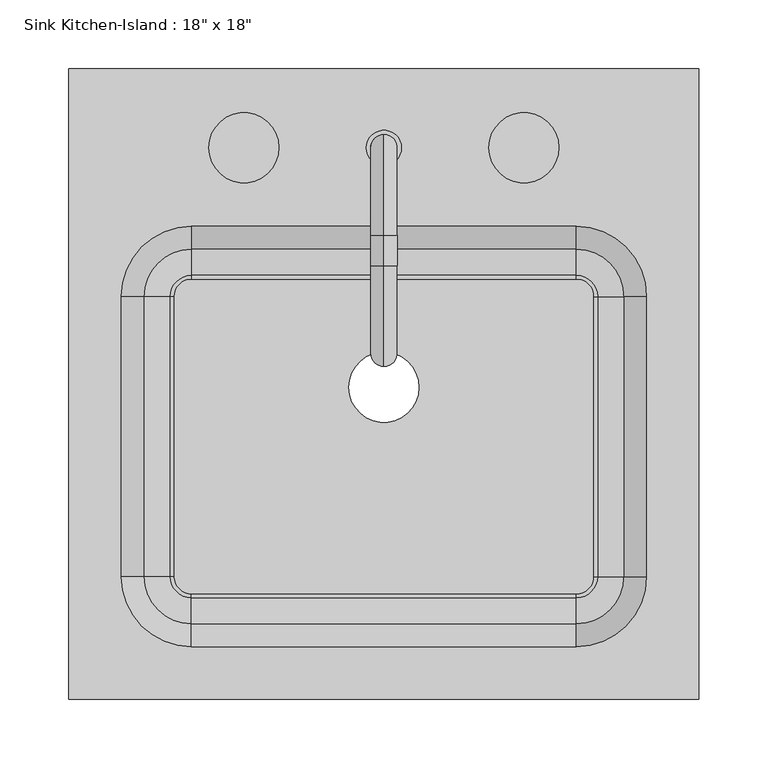
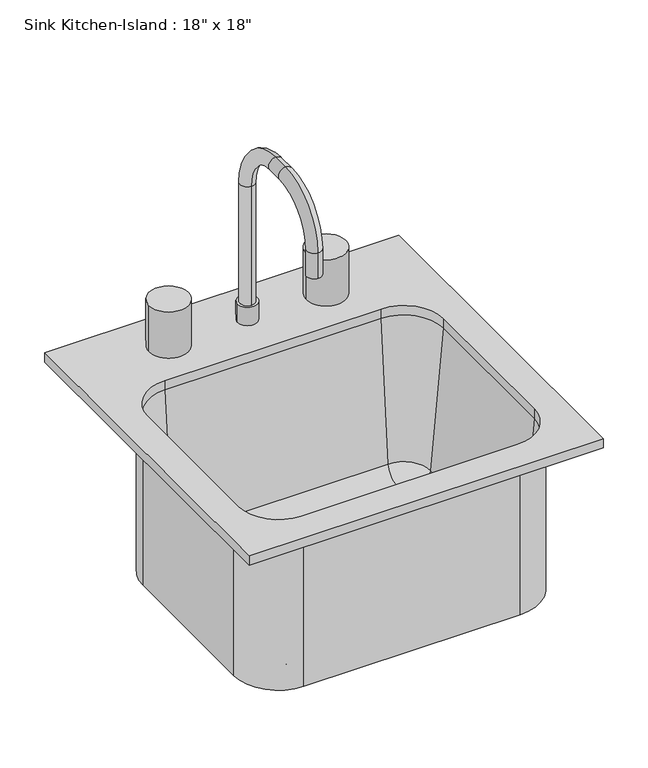
"""IFC4 building model written with IfcOpenShell, lengths in millimetres: flow terminal geometry."""

from ifc_helpers import new_model, si_unit, point, frame, frame_2d, origin, place, context, project, spatial, polyline, circle_curve, ellipse_curve, trimmed, segment, composite_curve, outline, extrude, source, transform, mapped, element, save
from ifc_brep_helpers import plane_surface, cylinder_surface, revolved_surface, advanced_brep


def flow_terminal_871c2e40(model_context):
    return source(origin(), model_context, "Body", "SolidModel", [
        advanced_brep(
        [(244.2892406, 230.9454011, 927.1), (-212.9107594, 230.9454011, 927.1), (-212.9107594, -226.2545989, 927.1), (244.2892406, -226.2545989, 927.1), (155.3892406, 116.6454011, 927.1), (206.1892406, 65.8454011, 927.1), (206.1892406, -137.3545989, 927.1), (155.3892406, -188.1545989, 927.1), (-124.0107594, -188.1545989, 927.1), (-174.8107594, -137.3545989, 927.1), (-174.8107594, 65.8454011, 927.1), (-124.0107594, 116.6454011, 927.1), (244.2892406, 230.9454011, 914.4), (244.2892406, -226.2545989, 914.4), (-212.9107594, -226.2545989, 914.4), (-212.9107594, 230.9454011, 914.4), (212.5392406, 65.8454011, 914.4), (155.3892406, 122.9954011, 914.4), (-124.0107594, 122.9954011, 914.4), (-181.1607594, 65.8454011, 914.4), (-181.1607594, -137.3545989, 914.4), (-124.0107594, -194.5045989, 914.4), (155.3892406, -194.5045989, 914.4), (212.5392406, -137.3545989, 914.4), (155.3892406, 116.6454011, 914.4), (206.1892406, 65.8454011, 914.4), (206.1892406, -137.3545989, 914.4), (155.3892406, -188.1545989, 914.4), (-124.0107594, -188.1545989, 914.4), (-174.8107594, -137.3545989, 914.4), (-174.8107594, 65.8454011, 914.4), (-124.0107594, 116.6454011, 914.4), (212.5392406, 65.8454011, 698.5), (155.3892406, 122.9954011, 698.5), (168.0892406, 65.8454011, 698.5), (155.3892406, 78.5454011, 698.5), (168.0892406, 65.8454011, 708.025), (155.3892406, 78.5454011, 708.025), (170.6776588, 65.8454011, 708.025), (155.3892406, 81.1338193, 708.025), (189.6551678, 65.8454011, 725.4146831), (155.3892406, 100.1113283, 725.4146831), (212.5392406, -137.3545989, 698.5), (168.0892406, -137.3545989, 698.5), (168.0892406, -137.3545989, 708.025), (170.6776588, -137.3545989, 708.025), (189.6551678, -137.3545989, 725.4146831), (155.3892406, -194.5045989, 698.5), (155.3892406, -150.0545989, 698.5), (155.3892406, -150.0545989, 708.025), (155.3892406, -152.6430171, 708.025), (155.3892406, -171.6205261, 725.4146831), (-124.0107594, -194.5045989, 698.5), (-124.0107594, -150.0545989, 698.5), (-124.0107594, -150.0545989, 708.025), (-124.0107594, -152.6430171, 708.025), (-124.0107594, -171.6205261, 725.4146831), (-181.1607594, -137.3545989, 698.5), (-136.7107594, -137.3545989, 698.5), (-136.7107594, -137.3545989, 708.025), (-139.2991776, -137.3545989, 708.025), (-158.2766866, -137.3545989, 725.4146831), (-181.1607594, 65.8454011, 698.5), (-136.7107594, 65.8454011, 698.5), (-136.7107594, 65.8454011, 708.025), (-139.2991776, 65.8454011, 708.025), (-158.2766866, 65.8454011, 725.4146831), (-124.0107594, 122.9954011, 698.5), (-124.0107594, 78.5454011, 698.5), (-124.0107594, 78.5454011, 708.025), (-124.0107594, 81.1338193, 708.025), (-124.0107594, 100.1113283, 725.4146831)],
        [
            (0, 1),
            (1, 2),
            (2, 3),
            (3, 0),
            (4, 5, circle_curve(frame((155.3892406, 65.8454011, 927.1), z_axis=(0.0, 0.0, -1.0), x_axis=(1.0, 0.0, 0.0)), 50.8)),
            (5, 6),
            (6, 7, circle_curve(frame((155.3892406, -137.3545989, 927.1), z_axis=(0.0, 0.0, -1.0), x_axis=(1.0, 0.0, 0.0)), 50.8)),
            (7, 8),
            (8, 9, circle_curve(frame((-124.0107594, -137.3545989, 927.1), z_axis=(0.0, 0.0, -1.0), x_axis=(1.0, 0.0, 0.0)), 50.8)),
            (9, 10),
            (10, 11, circle_curve(frame((-124.0107594, 65.8454011, 927.1), z_axis=(0.0, 0.0, -1.0), x_axis=(1.0, 0.0, 0.0)), 50.8)),
            (11, 4),
            (12, 13),
            (13, 14),
            (14, 15),
            (15, 12),
            (16, 17, circle_curve(frame((155.3892406, 65.8454011, 914.4), z_axis=(0.0, 0.0, 1.0), x_axis=(0.0, 1.0, 0.0)), 57.15)),
            (17, 18),
            (18, 19, circle_curve(frame((-124.0107594, 65.8454011, 914.4), z_axis=(0.0, 0.0, 1.0), x_axis=(-1.0, 0.0, 0.0)), 57.15)),
            (19, 20),
            (20, 21, circle_curve(frame((-124.0107594, -137.3545989, 914.4), z_axis=(0.0, 0.0, 1.0), x_axis=(0.0, -1.0, 0.0)), 57.15)),
            (21, 22),
            (22, 23, circle_curve(frame((155.3892406, -137.3545989, 914.4), z_axis=(0.0, 0.0, 1.0), x_axis=(1.0, 0.0, 0.0)), 57.15)),
            (23, 16),
            (0, 12),
            (15, 1),
            (14, 2),
            (13, 3),
            (4, 24),
            (24, 25, circle_curve(frame((155.3892406, 65.8454011, 914.4), z_axis=(0.0, 0.0, -1.0), x_axis=(1.0, 0.0, 0.0)), 50.8)),
            (25, 5),
            (25, 26),
            (26, 6),
            (26, 27, circle_curve(frame((155.3892406, -137.3545989, 914.4), z_axis=(0.0, 0.0, -1.0), x_axis=(1.0, 0.0, 0.0)), 50.8)),
            (27, 7),
            (27, 28),
            (28, 8),
            (28, 29, circle_curve(frame((-124.0107594, -137.3545989, 914.4), z_axis=(0.0, 0.0, -1.0), x_axis=(1.0, 0.0, 0.0)), 50.8)),
            (29, 9),
            (29, 30),
            (30, 10),
            (30, 31, circle_curve(frame((-124.0107594, 65.8454011, 914.4), z_axis=(0.0, 0.0, -1.0), x_axis=(1.0, 0.0, 0.0)), 50.8)),
            (31, 11),
            (31, 24),
            (32, 33, circle_curve(frame((155.3892406, 65.8454011, 698.5), z_axis=(0.0, 0.0, 1.0), x_axis=(0.0, 1.0, 0.0)), 57.15)),
            (33, 17),
            (16, 32),
            (32, 34),
            (34, 35, circle_curve(frame((155.3892406, 65.8454011, 698.5), z_axis=(0.0, 0.0, 1.0), x_axis=(0.0, 1.0, 0.0)), 12.7)),
            (35, 33),
            (34, 36),
            (36, 37, circle_curve(frame((155.3892406, 65.8454011, 708.025), z_axis=(0.0, 0.0, 1.0), x_axis=(0.0, 1.0, 0.0)), 12.7)),
            (37, 35),
            (36, 38),
            (38, 39, circle_curve(frame((155.3892406, 65.8454011, 708.025), z_axis=(0.0, 0.0, 1.0), x_axis=(0.0, 1.0, 0.0)), 15.2884182)),
            (39, 37),
            (38, 40, circle_curve(frame((170.6776588, 65.8454011, 727.075), z_axis=(0.0, -1.0, 0.0), x_axis=(1.0, 0.0, 0.0)), 19.05)),
            (40, 41, circle_curve(frame((155.3892406, 65.8454011, 725.4146831), z_axis=(0.0, 0.0, 1.0), x_axis=(0.0, 1.0, 0.0)), 34.2659272)),
            (41, 39, circle_curve(frame((155.3892406, 81.1338193, 727.075), z_axis=(-1.0, 0.0, 0.0), x_axis=(0.0, 1.0, 0.0)), 19.05)),
            (40, 25),
            (24, 41),
            (23, 42),
            (42, 32),
            (42, 43),
            (43, 34),
            (43, 44),
            (44, 36),
            (44, 45),
            (45, 38),
            (45, 46, circle_curve(frame((170.6776588, -137.3545989, 727.075), z_axis=(0.0, -1.0, 0.0), x_axis=(1.0, 0.0, 0.0)), 19.05)),
            (46, 40),
            (46, 26),
            (22, 47),
            (47, 42, circle_curve(frame((155.3892406, -137.3545989, 698.5), z_axis=(0.0, 0.0, 1.0), x_axis=(1.0, 0.0, 0.0)), 57.15)),
            (47, 48),
            (48, 43, circle_curve(frame((155.3892406, -137.3545989, 698.5), z_axis=(0.0, 0.0, 1.0), x_axis=(1.0, 0.0, 0.0)), 12.7)),
            (48, 49),
            (49, 44, circle_curve(frame((155.3892406, -137.3545989, 708.025), z_axis=(0.0, 0.0, 1.0), x_axis=(1.0, 0.0, 0.0)), 12.7)),
            (49, 50),
            (50, 45, circle_curve(frame((155.3892406, -137.3545989, 708.025), z_axis=(0.0, 0.0, 1.0), x_axis=(1.0, 0.0, 0.0)), 15.2884182)),
            (50, 51, circle_curve(frame((155.3892406, -152.6430171, 727.075), z_axis=(-1.0, 0.0, 0.0), x_axis=(0.0, -1.0, 0.0)), 19.05)),
            (51, 46, circle_curve(frame((155.3892406, -137.3545989, 725.4146831), z_axis=(0.0, 0.0, 1.0), x_axis=(1.0, 0.0, 0.0)), 34.2659272)),
            (51, 27),
            (21, 52),
            (52, 47),
            (52, 53),
            (53, 48),
            (53, 54),
            (54, 49),
            (54, 55),
            (55, 50),
            (55, 56, circle_curve(frame((-124.0107594, -152.6430171, 727.075), z_axis=(-1.0, 0.0, 0.0), x_axis=(0.0, -1.0, 0.0)), 19.05)),
            (56, 51),
            (56, 28),
            (20, 57),
            (57, 52, circle_curve(frame((-124.0107594, -137.3545989, 698.5), z_axis=(0.0, 0.0, 1.0), x_axis=(0.0, -1.0, 0.0)), 57.15)),
            (57, 58),
            (58, 53, circle_curve(frame((-124.0107594, -137.3545989, 698.5), z_axis=(0.0, 0.0, 1.0), x_axis=(0.0, -1.0, 0.0)), 12.7)),
            (58, 59),
            (59, 54, circle_curve(frame((-124.0107594, -137.3545989, 708.025), z_axis=(0.0, 0.0, 1.0), x_axis=(0.0, -1.0, 0.0)), 12.7)),
            (59, 60),
            (60, 55, circle_curve(frame((-124.0107594, -137.3545989, 708.025), z_axis=(0.0, 0.0, 1.0), x_axis=(0.0, -1.0, 0.0)), 15.2884182)),
            (60, 61, circle_curve(frame((-139.2991776, -137.3545989, 727.075), z_axis=(0.0, 1.0, 0.0), x_axis=(-1.0, 0.0, 0.0)), 19.05)),
            (61, 56, circle_curve(frame((-124.0107594, -137.3545989, 725.4146831), z_axis=(0.0, 0.0, 1.0), x_axis=(0.0, -1.0, 0.0)), 34.2659272)),
            (61, 29),
            (19, 62),
            (62, 57),
            (62, 63),
            (63, 58),
            (63, 64),
            (64, 59),
            (64, 65),
            (65, 60),
            (65, 66, circle_curve(frame((-139.2991776, 65.8454011, 727.075), z_axis=(0.0, 1.0, 0.0), x_axis=(-1.0, 0.0, 0.0)), 19.05)),
            (66, 61),
            (66, 30),
            (18, 67),
            (67, 62, circle_curve(frame((-124.0107594, 65.8454011, 698.5), z_axis=(0.0, 0.0, 1.0), x_axis=(-1.0, 0.0, 0.0)), 57.15)),
            (67, 68),
            (68, 63, circle_curve(frame((-124.0107594, 65.8454011, 698.5), z_axis=(0.0, 0.0, 1.0), x_axis=(-1.0, 0.0, 0.0)), 12.7)),
            (68, 69),
            (69, 64, circle_curve(frame((-124.0107594, 65.8454011, 708.025), z_axis=(0.0, 0.0, 1.0), x_axis=(-1.0, 0.0, 0.0)), 12.7)),
            (69, 70),
            (70, 65, circle_curve(frame((-124.0107594, 65.8454011, 708.025), z_axis=(0.0, 0.0, 1.0), x_axis=(-1.0, 0.0, 0.0)), 15.2884182)),
            (70, 71, circle_curve(frame((-124.0107594, 81.1338193, 727.075), z_axis=(1.0, 0.0, 0.0), x_axis=(0.0, 1.0, 0.0)), 19.05)),
            (71, 66, circle_curve(frame((-124.0107594, 65.8454011, 725.4146831), z_axis=(0.0, 0.0, 1.0), x_axis=(-1.0, 0.0, 0.0)), 34.2659272)),
            (71, 31),
            (33, 67),
            (35, 68),
            (37, 69),
            (39, 70),
            (41, 71),
        ],
        [
            plane_surface(frame((-212.9107594, 230.9454011, 927.1), z_axis=(0.0, 0.0, 1.0), x_axis=(-1.0, 0.0, 0.0))),
            plane_surface(frame((-212.9107594, 230.9454011, 914.4), z_axis=(0.0, 0.0, -1.0), x_axis=(1.0, 0.0, 0.0))),
            plane_surface(frame((244.2892406, 230.9454011, 927.1), z_axis=(0.0, 1.0, 0.0), x_axis=(0.0, 0.0, -1.0))),
            plane_surface(frame((-212.9107594, 230.9454011, 927.1), z_axis=(-1.0, 0.0, 0.0), x_axis=(0.0, 0.0, -1.0))),
            plane_surface(frame((-212.9107594, -226.2545989, 927.1), z_axis=(0.0, -1.0, 0.0), x_axis=(0.0, 0.0, -1.0))),
            plane_surface(frame((244.2892406, -226.2545989, 927.1), z_axis=(1.0, 0.0, 0.0), x_axis=(0.0, 0.0, -1.0))),
            revolved_surface(polyline([(206.1892406, 65.8454011, 914.4), (206.1892406, 65.8454011, 927.1)]), (155.3892406, 65.8454011, 0.0), (0.0, 0.0, -1.0)),
            plane_surface(frame((206.1892406, 65.8454011, 927.1), z_axis=(-1.0, 0.0, 0.0), x_axis=(0.0, 0.0, -1.0))),
            revolved_surface(polyline([(206.1892406, -137.3545989, 914.4), (206.1892406, -137.3545989, 927.1)]), (155.3892406, -137.3545989, 0.0), (0.0, 0.0, -1.0)),
            plane_surface(frame((155.3892406, -188.1545989, 927.1), z_axis=(0.0, 1.0, 0.0), x_axis=(0.0, 0.0, -1.0))),
            revolved_surface(polyline([(-73.2107594, -137.3545989, 914.4), (-73.2107594, -137.3545989, 927.1)]), (-124.0107594, -137.3545989, 0.0), (0.0, 0.0, -1.0)),
            plane_surface(frame((-174.8107594, -137.3545989, 927.1), z_axis=(1.0, 0.0, 0.0), x_axis=(0.0, 0.0, -1.0))),
            revolved_surface(polyline([(-73.2107594, 65.8454011, 914.4), (-73.2107594, 65.8454011, 927.1)]), (-124.0107594, 65.8454011, 0.0), (0.0, 0.0, -1.0)),
            plane_surface(frame((-124.0107594, 116.6454011, 927.1), z_axis=(0.0, -1.0, 0.0), x_axis=(0.0, 0.0, -1.0))),
            cylinder_surface(frame((155.3892406, 65.8454011, 0.0), z_axis=(0.0, 0.0, -1.0), x_axis=(0.0, 1.0, 0.0)), 57.15),
            plane_surface(frame((155.3892406, 65.8454011, 698.5), z_axis=(0.0, 0.0, -1.0), x_axis=(0.0, 1.0, 0.0))),
            revolved_surface(polyline([(155.3892406, 78.5454011, 698.5), (155.3892406, 78.5454011, 708.025)]), (155.3892406, 65.8454011, 0.0), (0.0, 0.0, -1.0)),
            plane_surface(frame((155.3892406, 65.8454011, 708.025), z_axis=(0.0, 0.0, 1.0), x_axis=(0.0, 1.0, 0.0))),
            revolved_surface(trimmed(ellipse_curve(frame((155.3892406, 81.1338193, 727.075), z_axis=(1.0, 0.0, 0.0), x_axis=(0.0, 1.0, 0.0)), 19.05, 19.05), [point((155.3892406, 81.1338193, 708.025))], [point((155.3892406, 100.1113283, 725.4146831))], True, "CARTESIAN"), (155.3892406, 65.8454011, 0.0), (0.0, 0.0, -1.0)),
            revolved_surface(polyline([(155.3892406, 100.1113283, 725.4146831), (155.3892406, 116.6454011, 914.4)]), (155.3892406, 65.8454011, 0.0), (0.0, 0.0, -1.0)),
            plane_surface(frame((212.5392406, 65.8454011, 914.4), z_axis=(1.0, 0.0, 0.0), x_axis=(0.0, -1.0, 0.0))),
            plane_surface(frame((212.5392406, 65.8454011, 698.5), z_axis=(0.0, 0.0, -1.0), x_axis=(0.0, -1.0, 0.0))),
            plane_surface(frame((168.0892406, 65.8454011, 698.5), z_axis=(-1.0, 0.0, 0.0), x_axis=(0.0, -1.0, 0.0))),
            plane_surface(frame((168.0892406, 65.8454011, 708.025), z_axis=(0.0, 0.0, 1.0), x_axis=(0.0, -1.0, 0.0))),
            revolved_surface(polyline([(189.7276588, -137.3545989, 727.075), (189.7276588, 65.8454011, 727.075)]), (170.6776588, 65.8454011, 727.075), (0.0, -1.0, 0.0)),
            plane_surface(frame((189.6551678, 65.8454011, 725.4146831), z_axis=(-0.9961946980917443, 0.0, 0.08715574274767254), x_axis=(0.0, -1.0, 0.0))),
            cylinder_surface(frame((155.3892406, -137.3545989, 0.0), z_axis=(0.0, 0.0, -1.0), x_axis=(1.0, 0.0, 0.0)), 57.15),
            plane_surface(frame((155.3892406, -137.3545989, 698.5), z_axis=(0.0, 0.0, -1.0), x_axis=(1.0, 0.0, 0.0))),
            revolved_surface(polyline([(168.08924059999998, -137.3545989, 698.5), (168.08924059999998, -137.3545989, 708.025)]), (155.3892406, -137.3545989, 0.0), (0.0, 0.0, -1.0)),
            plane_surface(frame((155.3892406, -137.3545989, 708.025), z_axis=(0.0, 0.0, 1.0), x_axis=(1.0, 0.0, 0.0))),
            revolved_surface(trimmed(ellipse_curve(frame((170.6776588, -137.3545989, 727.075), z_axis=(0.0, -1.0, 0.0), x_axis=(1.0, 0.0, 0.0)), 19.05, 19.05), [point((170.6776588, -137.3545989, 708.025))], [point((189.6551678, -137.3545989, 725.4146831))], True, "CARTESIAN"), (155.3892406, -137.3545989, 0.0), (0.0, 0.0, -1.0)),
            revolved_surface(polyline([(189.6551678, -137.3545989, 725.4146831), (206.1892406, -137.3545989, 914.4)]), (155.3892406, -137.3545989, 0.0), (0.0, 0.0, -1.0)),
            plane_surface(frame((155.3892406, -194.5045989, 914.4), z_axis=(0.0, -1.0, 0.0), x_axis=(-1.0, 0.0, 0.0))),
            plane_surface(frame((155.3892406, -194.5045989, 698.5), z_axis=(0.0, 0.0, -1.0), x_axis=(-1.0, 0.0, 0.0))),
            plane_surface(frame((155.3892406, -150.0545989, 698.5), z_axis=(0.0, 1.0, 0.0), x_axis=(-1.0, 0.0, 0.0))),
            plane_surface(frame((155.3892406, -150.0545989, 708.025), z_axis=(0.0, 0.0, 1.0), x_axis=(-1.0, 0.0, 0.0))),
            revolved_surface(polyline([(-124.01075939999998, -171.69301710000002, 727.075), (155.3892406, -171.69301710000002, 727.075)]), (155.3892406, -152.6430171, 727.075), (-1.0, 0.0, 0.0)),
            plane_surface(frame((155.3892406, -171.6205261, 725.4146831), z_axis=(0.0, 0.9961946980917443, 0.08715574274767254), x_axis=(-1.0, 0.0, 0.0))),
            cylinder_surface(frame((-124.0107594, -137.3545989, 0.0), z_axis=(0.0, 0.0, -1.0), x_axis=(0.0, -1.0, 0.0)), 57.15),
            plane_surface(frame((-124.0107594, -137.3545989, 698.5), z_axis=(0.0, 0.0, -1.0), x_axis=(0.0, -1.0, 0.0))),
            revolved_surface(polyline([(-124.0107594, -150.0545989, 698.5), (-124.0107594, -150.0545989, 708.025)]), (-124.0107594, -137.3545989, 0.0), (0.0, 0.0, -1.0)),
            plane_surface(frame((-124.0107594, -137.3545989, 708.025), z_axis=(0.0, 0.0, 1.0), x_axis=(0.0, -1.0, 0.0))),
            revolved_surface(trimmed(ellipse_curve(frame((-124.0107594, -152.6430171, 727.075), z_axis=(-1.0, 0.0, 0.0), x_axis=(0.0, -1.0, 0.0)), 19.05, 19.05), [point((-124.0107594, -152.6430171, 708.025))], [point((-124.0107594, -171.6205261, 725.4146831))], True, "CARTESIAN"), (-124.0107594, -137.3545989, 0.0), (0.0, 0.0, -1.0)),
            revolved_surface(polyline([(-124.0107594, -171.6205261, 725.4146831), (-124.0107594, -188.1545989, 914.4)]), (-124.0107594, -137.3545989, 0.0), (0.0, 0.0, -1.0)),
            plane_surface(frame((-181.1607594, -137.3545989, 914.4), z_axis=(-1.0, 0.0, 0.0), x_axis=(0.0, 1.0, 0.0))),
            plane_surface(frame((-181.1607594, -137.3545989, 698.5), z_axis=(0.0, 0.0, -1.0), x_axis=(0.0, 1.0, 0.0))),
            plane_surface(frame((-136.7107594, -137.3545989, 698.5), z_axis=(1.0, 0.0, 0.0), x_axis=(0.0, 1.0, 0.0))),
            plane_surface(frame((-136.7107594, -137.3545989, 708.025), z_axis=(0.0, 0.0, 1.0), x_axis=(0.0, 1.0, 0.0))),
            revolved_surface(polyline([(-158.34917760000002, 65.8454011, 727.075), (-158.34917760000002, -137.3545989, 727.075)]), (-139.2991776, -137.3545989, 727.075), (0.0, 1.0, 0.0)),
            plane_surface(frame((-158.2766866, -137.3545989, 725.4146831), z_axis=(0.9961946980917443, 0.0, 0.08715574274767254), x_axis=(0.0, 1.0, 0.0))),
            cylinder_surface(frame((-124.0107594, 65.8454011, 0.0), z_axis=(0.0, 0.0, -1.0), x_axis=(-1.0, 0.0, 0.0)), 57.15),
            plane_surface(frame((-124.0107594, 65.8454011, 698.5), z_axis=(0.0, 0.0, -1.0), x_axis=(-1.0, 0.0, 0.0))),
            revolved_surface(polyline([(-136.7107594, 65.8454011, 698.5), (-136.7107594, 65.8454011, 708.025)]), (-124.0107594, 65.8454011, 0.0), (0.0, 0.0, -1.0)),
            plane_surface(frame((-124.0107594, 65.8454011, 708.025), z_axis=(0.0, 0.0, 1.0), x_axis=(-1.0, 0.0, 0.0))),
            revolved_surface(trimmed(ellipse_curve(frame((-139.2991776, 65.8454011, 727.075), z_axis=(0.0, 1.0, 0.0), x_axis=(-1.0, 0.0, 0.0)), 19.05, 19.05), [point((-139.2991776, 65.8454011, 708.025))], [point((-158.2766866, 65.8454011, 725.4146831))], True, "CARTESIAN"), (-124.0107594, 65.8454011, 0.0), (0.0, 0.0, -1.0)),
            revolved_surface(polyline([(-158.2766866, 65.8454011, 725.4146831), (-174.8107594, 65.8454011, 914.4)]), (-124.0107594, 65.8454011, 0.0), (0.0, 0.0, -1.0)),
            plane_surface(frame((-124.0107594, 122.9954011, 914.4), z_axis=(0.0, 1.0, 0.0), x_axis=(1.0, 0.0, 0.0))),
            plane_surface(frame((-124.0107594, 122.9954011, 698.5), z_axis=(0.0, 0.0, -1.0), x_axis=(1.0, 0.0, 0.0))),
            plane_surface(frame((-124.0107594, 78.5454011, 698.5), z_axis=(0.0, -1.0, 0.0), x_axis=(1.0, 0.0, 0.0))),
            plane_surface(frame((-124.0107594, 78.5454011, 708.025), z_axis=(0.0, 0.0, 1.0), x_axis=(1.0, 0.0, 0.0))),
            revolved_surface(polyline([(155.3892406, 100.1838193, 727.075), (-124.0107594, 100.1838193, 727.075)]), (-124.0107594, 81.1338193, 727.075), (1.0, 0.0, 0.0)),
            plane_surface(frame((-124.0107594, 100.1113283, 725.4146831), z_axis=(0.0, -0.9961946980917443, 0.08715574274767254), x_axis=(1.0, 0.0, 0.0))),
        ],
        [
            (0, [[1, 2, 3, 4], [5, 6, 7, 8, 9, 10, 11, 12]]),
            (1, [[13, 14, 15, 16], [17, 18, 19, 20, 21, 22, 23, 24]]),
            (2, [[-1, 25, -16, 26]]),
            (3, [[-2, -26, -15, 27]]),
            (4, [[-3, -27, -14, 28]]),
            (5, [[-4, -28, -13, -25]]),
            (6, [[-5, 29, 30, 31]]),
            (7, [[-6, -31, 32, 33]]),
            (8, [[-7, -33, 34, 35]]),
            (9, [[-8, -35, 36, 37]]),
            (10, [[-9, -37, 38, 39]]),
            (11, [[-10, -39, 40, 41]]),
            (12, [[-11, -41, 42, 43]]),
            (13, [[-12, -43, 44, -29]]),
            (14, [[45, 46, -17, 47]]),
            (15, [[-45, 48, 49, 50]]),
            (16, [[-49, 51, 52, 53]]),
            (17, [[-52, 54, 55, 56]]),
            (18, [[-55, 57, 58, 59]]),
            (19, [[-58, 60, -30, 61]]),
            (20, [[-47, -24, 62, 63]]),
            (21, [[-48, -63, 64, 65]]),
            (22, [[-51, -65, 66, 67]]),
            (23, [[-54, -67, 68, 69]]),
            (24, [[-57, -69, 70, 71]]),
            (25, [[-60, -71, 72, -32]]),
            (26, [[-62, -23, 73, 74]]),
            (27, [[-64, -74, 75, 76]]),
            (28, [[-66, -76, 77, 78]]),
            (29, [[-68, -78, 79, 80]]),
            (30, [[-70, -80, 81, 82]]),
            (31, [[-72, -82, 83, -34]]),
            (32, [[-73, -22, 84, 85]]),
            (33, [[-75, -85, 86, 87]]),
            (34, [[-77, -87, 88, 89]]),
            (35, [[-79, -89, 90, 91]]),
            (36, [[-81, -91, 92, 93]]),
            (37, [[-83, -93, 94, -36]]),
            (38, [[-84, -21, 95, 96]]),
            (39, [[-86, -96, 97, 98]]),
            (40, [[-88, -98, 99, 100]]),
            (41, [[-90, -100, 101, 102]]),
            (42, [[-92, -102, 103, 104]]),
            (43, [[-94, -104, 105, -38]]),
            (44, [[-95, -20, 106, 107]]),
            (45, [[-97, -107, 108, 109]]),
            (46, [[-99, -109, 110, 111]]),
            (47, [[-101, -111, 112, 113]]),
            (48, [[-103, -113, 114, 115]]),
            (49, [[-105, -115, 116, -40]]),
            (50, [[-106, -19, 117, 118]]),
            (51, [[-108, -118, 119, 120]]),
            (52, [[-110, -120, 121, 122]]),
            (53, [[-112, -122, 123, 124]]),
            (54, [[-114, -124, 125, 126]]),
            (55, [[-116, -126, 127, -42]]),
            (56, [[-46, 128, -117, -18]]),
            (57, [[-50, 129, -119, -128]]),
            (58, [[-53, 130, -121, -129]]),
            (59, [[-56, 131, -123, -130]]),
            (60, [[-59, 132, -125, -131]]),
            (61, [[-61, -44, -127, -132]]),
        ],
    ),
        advanced_brep(
        [(2.9892406, 173.7954011, 927.1), (28.3892406, 173.7954011, 927.1), (15.6892406, 183.3204011, 1114.425), (15.6892406, 164.2704011, 1114.425), (15.6892406, 164.2704011, 952.5), (15.6892406, 183.3204011, 952.5), (15.6892406, 110.2954011, 1187.45), (15.6892406, 110.2954011, 1168.4), (15.6892406, 88.0704011, 1187.45), (15.6892406, 88.0704011, 1168.4), (15.6892406, 15.0454011, 1114.425), (15.6892406, 34.0954011, 1114.425), (15.6892406, 15.0454011, 1079.5), (15.6892406, 34.0954011, 1079.5), (2.9892406, 173.7954011, 952.5), (28.3892406, 173.7954011, 952.5)],
        [
            (0, 1, circle_curve(frame((15.6892406, 173.7954011, 927.1), z_axis=(0.0, 0.0, -1.0), x_axis=(1.0, 0.0, 0.0)), 12.7)),
            (1, 0, circle_curve(frame((15.6892406, 173.7954011, 927.1), z_axis=(0.0, 0.0, -1.0), x_axis=(1.0, 0.0, 0.0)), 12.7)),
            (2, 3, circle_curve(frame((15.6892406, 173.7954011, 1114.425), z_axis=(0.0, 0.0, -1.0), x_axis=(0.0, -1.0, 0.0)), 9.525)),
            (3, 4),
            (4, 5, circle_curve(frame((15.6892406, 173.7954011, 952.5), z_axis=(0.0, 0.0, 1.0), x_axis=(0.0, -1.0, 0.0)), 9.525)),
            (5, 2),
            (3, 2, circle_curve(frame((15.6892406, 173.7954011, 1114.425), z_axis=(0.0, 0.0, -1.0), x_axis=(0.0, -1.0, 0.0)), 9.525)),
            (5, 4, circle_curve(frame((15.6892406, 173.7954011, 952.5), z_axis=(0.0, 0.0, 1.0), x_axis=(0.0, -1.0, 0.0)), 9.525)),
            (2, 6, circle_curve(frame((15.6892406, 110.2954011, 1114.425), z_axis=(1.0, 0.0, 0.0), x_axis=(0.0, 1.0, 0.0)), 73.025)),
            (6, 7, circle_curve(frame((15.6892406, 110.2954011, 1177.925), z_axis=(0.0, 1.0, 0.0), x_axis=(0.0, 0.0, -1.0)), 9.525)),
            (7, 3, circle_curve(frame((15.6892406, 110.2954011, 1114.425), z_axis=(-1.0, 0.0, 0.0), x_axis=(0.0, 1.0, 0.0)), 53.975)),
            (7, 6, circle_curve(frame((15.6892406, 110.2954011, 1177.925), z_axis=(0.0, 1.0, 0.0), x_axis=(0.0, 0.0, -1.0)), 9.525)),
            (6, 8),
            (8, 9, circle_curve(frame((15.6892406, 88.0704011, 1177.925), z_axis=(0.0, 1.0, 0.0), x_axis=(0.0, 0.0, -1.0)), 9.525)),
            (9, 7),
            (9, 8, circle_curve(frame((15.6892406, 88.0704011, 1177.925), z_axis=(0.0, 1.0, 0.0), x_axis=(0.0, 0.0, -1.0)), 9.525)),
            (8, 10, circle_curve(frame((15.6892406, 88.0704011, 1114.425), z_axis=(1.0, 0.0, 0.0), x_axis=(0.0, 0.0, 1.0)), 73.025)),
            (10, 11, circle_curve(frame((15.6892406, 24.5704011, 1114.425), z_axis=(0.0, 0.0, 1.0), x_axis=(0.0, 1.0, 0.0)), 9.525)),
            (11, 9, circle_curve(frame((15.6892406, 88.0704011, 1114.425), z_axis=(-1.0, 0.0, 0.0), x_axis=(0.0, 0.0, 1.0)), 53.975)),
            (11, 10, circle_curve(frame((15.6892406, 24.5704011, 1114.425), z_axis=(0.0, 0.0, 1.0), x_axis=(0.0, 1.0, 0.0)), 9.525)),
            (12, 13, circle_curve(frame((15.6892406, 24.5704011, 1079.5), z_axis=(0.0, 0.0, -1.0), x_axis=(0.0, 1.0, 0.0)), 9.525)),
            (13, 12, circle_curve(frame((15.6892406, 24.5704011, 1079.5), z_axis=(0.0, 0.0, -1.0), x_axis=(0.0, 1.0, 0.0)), 9.525)),
            (10, 12),
            (13, 11),
            (14, 15, circle_curve(frame((15.6892406, 173.7954011, 952.5), z_axis=(0.0, 0.0, 1.0), x_axis=(1.0, 0.0, 0.0)), 12.7)),
            (15, 14, circle_curve(frame((15.6892406, 173.7954011, 952.5), z_axis=(0.0, 0.0, 1.0), x_axis=(1.0, 0.0, 0.0)), 12.7)),
            (14, 0),
            (1, 15),
        ],
        [
            plane_surface(frame((15.6892406, 164.2704011, 927.1), z_axis=(0.0, 0.0, -1.0), x_axis=(1.0, 0.0, 0.0))),
            cylinder_surface(frame((15.6892406, 173.7954011, 927.1), z_axis=(0.0, 0.0, -1.0), x_axis=(0.0, -1.0, 0.0)), 9.525),
            revolved_surface(trimmed(ellipse_curve(frame((15.6892406, 173.7954011, 1114.425), z_axis=(0.0, 0.0, -1.0), x_axis=(0.0, -1.0, 0.0)), 9.525, 9.525), [point((15.6892406, 183.3204011, 1114.425))], [point((15.6892406, 164.2704011, 1114.425))], True, "CARTESIAN"), (15.6892406, 110.2954011, 1114.425), (1.0, 0.0, 0.0)),
            revolved_surface(trimmed(ellipse_curve(frame((15.6892406, 173.7954011, 1114.425), z_axis=(0.0, 0.0, -1.0), x_axis=(0.0, -1.0, 0.0)), 9.525, 9.525), [point((15.6892406, 164.2704011, 1114.425))], [point((15.6892406, 183.3204011, 1114.425))], True, "CARTESIAN"), (15.6892406, 110.2954011, 1114.425), (1.0, 0.0, 0.0)),
            cylinder_surface(frame((15.6892406, 110.2954011, 1177.925), z_axis=(0.0, 1.0, 0.0), x_axis=(0.0, 0.0, -1.0)), 9.525),
            revolved_surface(trimmed(ellipse_curve(frame((15.6892406, 88.0704011, 1177.925), z_axis=(0.0, 1.0, 0.0), x_axis=(0.0, 0.0, -1.0)), 9.525, 9.525), [point((15.6892406, 88.0704011, 1187.45))], [point((15.6892406, 88.0704011, 1168.4))], True, "CARTESIAN"), (15.6892406, 88.0704011, 1114.425), (1.0, 0.0, 0.0)),
            revolved_surface(trimmed(ellipse_curve(frame((15.6892406, 88.0704011, 1177.925), z_axis=(0.0, 1.0, 0.0), x_axis=(0.0, 0.0, -1.0)), 9.525, 9.525), [point((15.6892406, 88.0704011, 1168.4))], [point((15.6892406, 88.0704011, 1187.45))], True, "CARTESIAN"), (15.6892406, 88.0704011, 1114.425), (1.0, 0.0, 0.0)),
            plane_surface(frame((15.6892406, 15.0454011, 1079.5), z_axis=(0.0, 0.0, -1.0), x_axis=(-1.0, 0.0, 0.0))),
            cylinder_surface(frame((15.6892406, 24.5704011, 1114.425), z_axis=(0.0, 0.0, 1.0), x_axis=(0.0, 1.0, 0.0)), 9.525),
            plane_surface(frame((28.3892406, 173.7954011, 952.5), z_axis=(0.0, 0.0, 1.0), x_axis=(0.0, 1.0, 0.0))),
            cylinder_surface(frame((15.6892406, 173.7954011, 927.1), z_axis=(0.0, 0.0, 1.0), x_axis=(1.0, 0.0, 0.0)), 12.7),
        ],
        [
            (0, [[1, 2]]),
            (1, [[3, 4, 5, 6]]),
            (1, [[7, -6, 8, -4]]),
            (2, [[-3, 9, 10, 11]]),
            (3, [[-7, -11, 12, -9]]),
            (4, [[-10, 13, 14, 15]]),
            (4, [[-12, -15, 16, -13]]),
            (5, [[-14, 17, 18, 19]]),
            (6, [[-16, -19, 20, -17]]),
            (7, [[21, 22]]),
            (8, [[-18, 23, -22, 24]]),
            (8, [[-20, -24, -21, -23]]),
            (9, [[25, 26], [-5, -8]]),
            (10, [[-25, 27, -2, 28]]),
            (10, [[-26, -28, -1, -27]]),
        ],
    ),
        extrude(outline(composite_curve([segment(trimmed(circle_curve(frame_2d((-85.9107594, 173.7954011)), 25.4), [point((-111.3107594, 173.7954011))], [point((-60.5107594, 173.7954011))], False, "CARTESIAN"), True, "CONTINUOUS"), segment(trimmed(circle_curve(frame_2d((-85.9107594, 173.7954011)), 25.4), [point((-60.5107594, 173.7954011))], [point((-111.3107594, 173.7954011))], False, "CARTESIAN"), True, "CONTINUOUS")], self_intersect=False)), frame((0.0, 0.0, 927.1), z_axis=(0.0, 0.0, 1.0), x_axis=(1.0, 0.0, 0.0)), (0.0, 0.0, 1.0), 63.5),
        extrude(outline(composite_curve([segment(trimmed(circle_curve(frame_2d((117.2892406, 173.7954011)), 25.4), [point((91.8892406, 173.7954011))], [point((142.6892406, 173.7954011))], False, "CARTESIAN"), True, "CONTINUOUS"), segment(trimmed(circle_curve(frame_2d((117.2892406, 173.7954011)), 25.4), [point((142.6892406, 173.7954011))], [point((91.8892406, 173.7954011))], False, "CARTESIAN"), True, "CONTINUOUS")], self_intersect=False)), frame((0.0, 0.0, 927.1), z_axis=(0.0, 0.0, 1.0), x_axis=(1.0, 0.0, 0.0)), (0.0, 0.0, 1.0), 63.5),
        extrude(outline(composite_curve([segment(trimmed(circle_curve(frame_2d((155.3892406, 65.8454011)), 12.7), [point((155.3892406, 78.5454011))], [point((168.0892406, 65.8454011))], False, "CARTESIAN"), True, "CONTINUOUS"), segment(polyline([(168.0892406, 65.8454011), (168.0892406, -137.3545989)]), True, "CONTINUOUS"), segment(trimmed(circle_curve(frame_2d((155.3892406, -137.3545989)), 12.7), [point((168.0892406, -137.3545989))], [point((155.3892406, -150.0545989))], False, "CARTESIAN"), True, "CONTINUOUS"), segment(polyline([(155.3892406, -150.0545989), (-124.0107594, -150.0545989)]), True, "CONTINUOUS"), segment(trimmed(circle_curve(frame_2d((-124.0107594, -137.3545989)), 12.7), [point((-124.0107594, -150.0545989))], [point((-136.7107594, -137.3545989))], False, "CARTESIAN"), True, "CONTINUOUS"), segment(polyline([(-136.7107594, -137.3545989), (-136.7107594, 65.8454011)]), True, "CONTINUOUS"), segment(trimmed(circle_curve(frame_2d((-124.0107594, 65.8454011)), 12.7), [point((-136.7107594, 65.8454011))], [point((-124.0107594, 78.5454011))], False, "CARTESIAN"), True, "CONTINUOUS"), segment(polyline([(-124.0107594, 78.5454011), (155.3892406, 78.5454011)]), True, "CONTINUOUS")], self_intersect=False), holes=[composite_curve([segment(trimmed(circle_curve(frame_2d((15.6892406, 0.0)), 25.4), [point((-9.7107594, 0.0))], [point((41.0892406, 0.0))], True, "CARTESIAN"), True, "CONTINUOUS"), segment(trimmed(circle_curve(frame_2d((15.6892406, 0.0)), 25.4), [point((41.0892406, 0.0))], [point((-9.7107594, 0.0))], True, "CARTESIAN"), True, "CONTINUOUS")], self_intersect=False)]), frame((0.0, 0.0, 698.5), z_axis=(0.0, 0.0, 1.0), x_axis=(1.0, 0.0, 0.0)), (0.0, 0.0, 1.0), 9.525),
    ])


if __name__ == "__main__":
    model = new_model("IFC4")
    model_context = context("Model", 3, world=origin())
    ifc_project = project(units=[si_unit("LENGTHUNIT", "METRE", prefix="MILLI")], contexts=[model_context])
    site = spatial("IfcSite", under=ifc_project)
    building = spatial("IfcBuilding", under=site)
    placement = place(None, origin())
    flow_terminal_shape = flow_terminal_871c2e40(model_context)
    element("IfcFlowTerminal", 1, ObjectType="Sink Kitchen-Island : 18\" x 18\"", at=placement, inside=building, context=model_context, shape_type="MappedRepresentation", body=[
        mapped(flow_terminal_shape, transform((0.0, 0.0, 0.0), x_axis=(1.0, 0.0, 0.0), y_axis=(0.0, 1.0, 0.0), z_axis=(0.0, 0.0, 1.0))),
    ])
    save(model, "model.ifc")

# Revit data of these elements
# Type "Sink Kitchen-Island : 18\" x 18\""
#   Assembly Code = "D2010410"
#   Counter Height = 3' - 0"
#   Depth = 1' - 6"
#   Width = 1' - 6"
#   Faucet Material = Steel, Polished
#   Sink Material = Steel, Polished
#   Default Elevation = 0
# Element 1 (IfcFlowTerminal, "Sink Kitchen-Island : 18\" x 18\"")
#   Materials on its faces: "Steel, Polished"
# Materials
#   "Steel, Polished": class "Metal", colour RGB 192 192 192, transparency 0, Description = "Polished steel", Cost = 0
